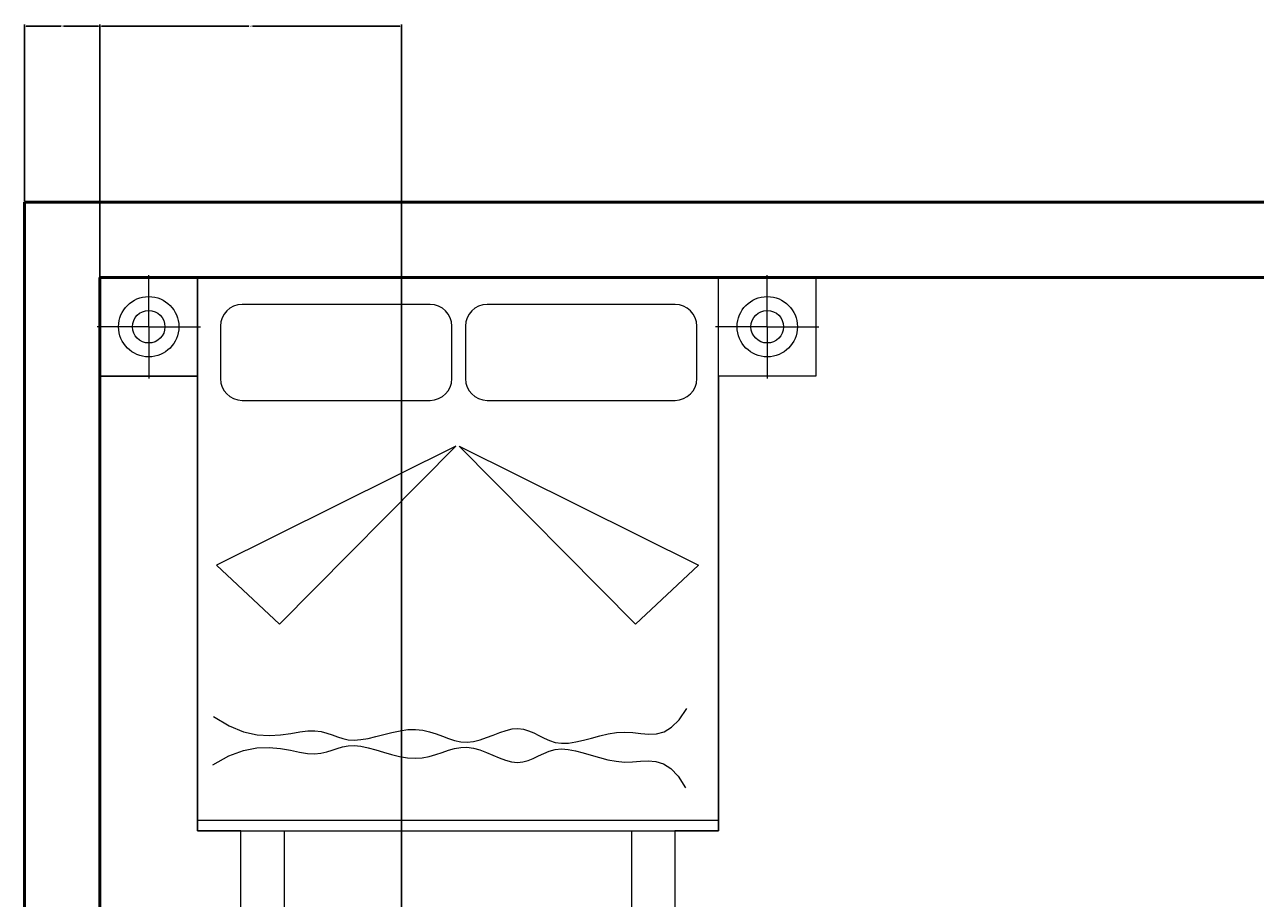
# Model space of a CAD drawing. Units: inches. Extents: x 1798 to 2141, y 1923 to 2386.
# Tile 6 of 9: x 1820 to 1967, y 2281 to 2386. Entities that reach past the tile are written whole.
import ezdxf

# ---------------------------------------------------------------- set-up
doc = ezdxf.new("R2010")
doc.units = ezdxf.units.IN
for name, color, linetype, lineweight in [('A-ANNO-DIMS', 2, 'Continuous', 18), ('A-FURN', 8, 'Continuous', 13), ('wall', 4, 'Continuous', 50)]:
    doc.layers.add(name, color=color, linetype=linetype, lineweight=lineweight)
doc.styles.get("Standard").update_dxf_attribs({"font": 'arial.ttf'})
doc.dimstyles.get("Standard").update_dxf_attribs({"dimtxt": 0.18, "dimasz": 0.18, "dimexe": 0.18, "dimexo": 0.0625, "dimgap": 0.09, "dimtad": 0, "dimtih": 1, "dimtoh": 1, "dimdec": 4, "dimzin": 0, "dimdsep": 46, "dimtxsty": 'Standard', "dimcen": 0.09, "dimadec": 0, "dimazin": 0, "dimtfac": 1, "dimtdec": 4, "dimtofl": 0, "dimtmove": 0, "dimatfit": 3, "dimfxl": 1, "dimtolj": 1, "dimtzin": 0, "dimarcsym": 0})

# ---------------------------------------------------------------- blocks, each defined once
blk = doc.blocks.new('A$C4F543DC7')
for p, q in [((0.0134, 3.35, -0.1688), (3.3134, 3.35, -0.1688)), ((0.4634, 3.35, -0.1688), (0.0134, 3.35, -0.1688)), ((0.0134, 2.896, -0.1688), (0.0134, 3.35, -0.1688)), ((0.0134, 3.35, -0.1688), (0.0134, 2.896, -0.1688)), ((0.2381, 3.1233, -0.4388), (0.2381, 3.3614, -0.4388)), ((0.4634, 3.35, -0.1688), (0.4634, 0.8, -0.1688)), ((2.8634, 3.35, -0.1688), (0.4634, 3.35, -0.1688)), ((0.4634, 2.896, -0.1688), (0.4634, 3.35, -0.1688)), ((2.8634, 0.8, -0.1688), (2.8634, 3.35, -0.1688)), ((2.8634, 3.35, -0.1688), (3.3134, 3.35, -0.1688)), ((2.8634, 2.896, -0.1688), (2.8634, 3.35, -0.1688)), ((3.0888, 3.1233, -0.4388), (3.0888, 3.3614, -0.4388)), ((3.3134, 3.35, -0.1688), (3.3134, 2.896, -0.1688)), ((3.3134, 3.35, -0.1688), (3.3134, 2.896, -0.1688)), ((1.5354, 3.226, -0.1688), (0.6684, 3.226, -0.1688)), ((2.6644, 3.226, -0.1688), (1.7974, 3.226, -0.1688)), ((0.2381, 3.1233, -0.4388), (0, 3.1233, -0.4388)), ((0.2381, 3.1233, -0.4388), (0.4762, 3.1233, -0.4388)), ((0.2381, 3.1233, -0.4388), (0.2381, 2.8852, -0.4388)), ((0.5684, 3.126, -0.1688), (0.5684, 2.884, -0.1688)), ((1.6354, 2.884, -0.1688), (1.6354, 3.126, -0.1688)), ((1.6974, 3.126, -0.1688), (1.6974, 2.884, -0.1688)), ((2.7644, 2.884, -0.1688), (2.7644, 3.126, -0.1688)), ((3.0888, 3.1233, -0.4388), (2.8507, 3.1233, -0.4388)), ((3.0888, 3.1233, -0.4388), (3.0888, 2.8852, -0.4388)), ((3.0888, 3.1233, -0.4388), (3.3269, 3.1233, -0.4388)), ((0.4634, 2.896, -0.1688), (0.0134, 2.896, -0.1688)), ((0.0134, 2.896, -0.1688), (0.4634, 2.896, -0.1688)), ((0.4634, 0.8, -0.1688), (0.4634, 2.896, -0.1688)), ((2.8634, 2.896, -0.1688), (2.8634, 0.8, -0.1688)), ((3.3134, 2.896, -0.1688), (2.8634, 2.896, -0.1688)), ((3.3134, 2.896, -0.1688), (2.8634, 2.896, -0.1688)), ((0.6684, 2.784, -0.1688), (1.5354, 2.784, -0.1688)), ((1.7974, 2.784, -0.1688), (2.6644, 2.784, -0.1688)), ((1.6534, 2.573, -0.1688), (0.5504, 2.025, -0.1688)), ((0.8414, 1.752, -0.1688), (1.6534, 2.573, -0.1688)), ((2.4814, 1.752, -0.1688), (1.6694, 2.573, -0.1688)), ((1.6694, 2.573, -0.1688), (2.7724, 2.025, -0.1688)), ((0.5504, 2.025, -0.1688), (0.8414, 1.752, -0.1688)), ((2.7724, 2.025, -0.1688), (2.4814, 1.752, -0.1688)), ((2.683, 1.312, -0.1688), (2.7182, 1.3641, -0.1688)), ((0.5369, 1.3267, -0.1688), (0.6088, 1.2835, -0.1688)), ((2.6479, 1.2774, -0.1688), (2.683, 1.312, -0.1688)), ((0.6088, 1.2835, -0.1688), (0.6756, 1.2566, -0.1688)), ((0.6756, 1.2566, -0.1688), (0.7373, 1.2428, -0.1688)), ((0.8457, 1.242, -0.1688), (0.8925, 1.2489, -0.1688)), ((0.8925, 1.2489, -0.1688), (0.9345, 1.2564, -0.1688)), ((0.9345, 1.2564, -0.1688), (0.9718, 1.2615, -0.1688)), ((0.9718, 1.2615, -0.1688), (1.0044, 1.2617, -0.1688)), ((1.0044, 1.2617, -0.1688), (1.0334, 1.2578, -0.1688)), ((1.0334, 1.2578, -0.1688), (1.0597, 1.2509, -0.1688)), ((1.0597, 1.2509, -0.1688), (1.0842, 1.2424, -0.1688)), ((1.3218, 1.2441, -0.1688), (1.3591, 1.2533, -0.1688)), ((1.3591, 1.2533, -0.1688), (1.3963, 1.2612, -0.1688)), ((1.3963, 1.2612, -0.1688), (1.4328, 1.2664, -0.1688)), ((1.4328, 1.2664, -0.1688), (1.4679, 1.2677, -0.1688)), ((1.4679, 1.2677, -0.1688), (1.501, 1.2643, -0.1688)), ((1.501, 1.2643, -0.1688), (1.5324, 1.257, -0.1688)), ((1.5324, 1.257, -0.1688), (1.5624, 1.2473, -0.1688)), ((1.8258, 1.2417, -0.1688), (1.8557, 1.2531, -0.1688)), ((1.8557, 1.2531, -0.1688), (1.8849, 1.263, -0.1688)), ((1.8849, 1.263, -0.1688), (1.913, 1.2698, -0.1688)), ((1.913, 1.2698, -0.1688), (1.9397, 1.2722, -0.1688)), ((1.9397, 1.2722, -0.1688), (1.9649, 1.2692, -0.1688)), ((1.9649, 1.2692, -0.1688), (1.989, 1.2617, -0.1688)), ((1.989, 1.2617, -0.1688), (2.0124, 1.2512, -0.1688)), ((2.0124, 1.2512, -0.1688), (2.0359, 1.2391, -0.1688)), ((2.3558, 1.2465, -0.1688), (2.3944, 1.2527, -0.1688)), ((2.3944, 1.2527, -0.1688), (2.4325, 1.255, -0.1688)), ((2.4325, 1.255, -0.1688), (2.4698, 1.2529, -0.1688)), ((2.4698, 1.2529, -0.1688), (2.5064, 1.2488, -0.1688)), ((2.5064, 1.2488, -0.1688), (2.5423, 1.2459, -0.1688)), ((2.5777, 1.2476, -0.1688), (2.6129, 1.257, -0.1688)), ((2.6129, 1.257, -0.1688), (2.6479, 1.2774, -0.1688)), ((0.7373, 1.2428, -0.1688), (0.794, 1.239, -0.1688)), ((0.794, 1.239, -0.1688), (0.8457, 1.242, -0.1688)), ((1.0842, 1.2424, -0.1688), (1.1081, 1.2336, -0.1688)), ((1.1081, 1.2336, -0.1688), (1.1322, 1.2257, -0.1688)), ((1.1316, 1.1872, -0.1688), (1.1573, 1.192, -0.1688)), ((1.1322, 1.2257, -0.1688), (1.1577, 1.2201, -0.1688)), ((1.1573, 1.192, -0.1688), (1.1851, 1.1932, -0.1688)), ((1.1577, 1.2201, -0.1688), (1.1855, 1.218, -0.1688)), ((1.1851, 1.1932, -0.1688), (1.2158, 1.1898, -0.1688)), ((1.1855, 1.218, -0.1688), (1.2163, 1.2204, -0.1688)), ((1.2163, 1.2204, -0.1688), (1.2498, 1.2264, -0.1688)), ((1.2498, 1.2264, -0.1688), (1.2852, 1.2347, -0.1688)), ((1.2852, 1.2347, -0.1688), (1.3218, 1.2441, -0.1688)), ((1.5624, 1.2473, -0.1688), (1.5915, 1.2365, -0.1688)), ((1.5915, 1.2365, -0.1688), (1.6199, 1.2259, -0.1688)), ((1.6199, 1.2259, -0.1688), (1.6481, 1.2169, -0.1688)), ((1.6481, 1.2169, -0.1688), (1.6765, 1.2108, -0.1688)), ((1.6765, 1.2108, -0.1688), (1.7053, 1.209, -0.1688)), ((1.7053, 1.209, -0.1688), (1.7349, 1.2124, -0.1688)), ((1.7349, 1.2124, -0.1688), (1.7651, 1.2199, -0.1688)), ((1.7651, 1.2199, -0.1688), (1.7955, 1.2301, -0.1688)), ((1.7955, 1.2301, -0.1688), (1.8258, 1.2417, -0.1688)), ((2.0359, 1.2391, -0.1688), (2.0599, 1.2269, -0.1688)), ((2.0599, 1.2269, -0.1688), (2.0849, 1.216, -0.1688)), ((2.0849, 1.216, -0.1688), (2.1117, 1.2077, -0.1688)), ((2.1117, 1.2077, -0.1688), (2.1407, 1.2037, -0.1688)), ((2.1407, 1.2037, -0.1688), (2.1723, 1.2047, -0.1688)), ((2.1723, 1.2047, -0.1688), (2.2062, 1.21, -0.1688)), ((2.2062, 1.21, -0.1688), (2.242, 1.2182, -0.1688)), ((2.242, 1.2182, -0.1688), (2.2791, 1.2279, -0.1688)), ((2.2791, 1.2279, -0.1688), (2.3173, 1.2378, -0.1688)), ((2.3173, 1.2378, -0.1688), (2.3558, 1.2465, -0.1688)), ((2.5423, 1.2459, -0.1688), (2.5777, 1.2476, -0.1688)), ((0.5334, 1.105, -0.1688), (0.6067, 1.1458, -0.1688)), ((0.6067, 1.1458, -0.1688), (0.6743, 1.1706, -0.1688)), ((0.6743, 1.1706, -0.1688), (0.7364, 1.1825, -0.1688)), ((0.7364, 1.1825, -0.1688), (0.7931, 1.1846, -0.1688)), ((0.7931, 1.1846, -0.1688), (0.8447, 1.1799, -0.1688)), ((0.8447, 1.1799, -0.1688), (0.8913, 1.1716, -0.1688)), ((0.8913, 1.1716, -0.1688), (0.9331, 1.1628, -0.1688)), ((0.9331, 1.1628, -0.1688), (0.9701, 1.1565, -0.1688)), ((0.9701, 1.1565, -0.1688), (1.0027, 1.1552, -0.1688)), ((1.0027, 1.1552, -0.1688), (1.0318, 1.1582, -0.1688)), ((1.0318, 1.1582, -0.1688), (1.0583, 1.1642, -0.1688)), ((1.0583, 1.1642, -0.1688), (1.0831, 1.172, -0.1688)), ((1.0831, 1.172, -0.1688), (1.1072, 1.18, -0.1688)), ((1.1072, 1.18, -0.1688), (1.1316, 1.1872, -0.1688)), ((1.2158, 1.1898, -0.1688), (1.2491, 1.1828, -0.1688)), ((1.2491, 1.1828, -0.1688), (1.2842, 1.1734, -0.1688)), ((1.2842, 1.1734, -0.1688), (1.3206, 1.1629, -0.1688)), ((1.3206, 1.1629, -0.1688), (1.3575, 1.1524, -0.1688)), ((1.3575, 1.1524, -0.1688), (1.3945, 1.1434, -0.1688)), ((1.3945, 1.1434, -0.1688), (1.4308, 1.1371, -0.1688)), ((1.4308, 1.1371, -0.1688), (1.4658, 1.1347, -0.1688)), ((1.4658, 1.1347, -0.1688), (1.499, 1.137, -0.1688)), ((1.499, 1.137, -0.1688), (1.5306, 1.1433, -0.1688)), ((1.5306, 1.1433, -0.1688), (1.5609, 1.152, -0.1688)), ((1.5609, 1.152, -0.1688), (1.5903, 1.1619, -0.1688)), ((1.5903, 1.1619, -0.1688), (1.6191, 1.1716, -0.1688)), ((1.6191, 1.1716, -0.1688), (1.6475, 1.1797, -0.1688)), ((1.6475, 1.1797, -0.1688), (1.676, 1.1849, -0.1688)), ((1.676, 1.1849, -0.1688), (1.7049, 1.1858, -0.1688)), ((1.7049, 1.1858, -0.1688), (1.7344, 1.1816, -0.1688)), ((1.7344, 1.1816, -0.1688), (1.7643, 1.1731, -0.1688)), ((1.7643, 1.1731, -0.1688), (1.7944, 1.1619, -0.1688)), ((1.7944, 1.1619, -0.1688), (1.8244, 1.1494, -0.1688)), ((1.8244, 1.1494, -0.1688), (1.8539, 1.137, -0.1688)), ((1.8539, 1.137, -0.1688), (1.8827, 1.1263, -0.1688)), ((2.0106, 1.134, -0.1688), (2.0344, 1.1454, -0.1688)), ((2.0344, 1.1454, -0.1688), (2.0588, 1.1568, -0.1688)), ((2.0588, 1.1568, -0.1688), (2.0842, 1.167, -0.1688)), ((2.0842, 1.167, -0.1688), (2.1112, 1.1743, -0.1688)), ((2.1112, 1.1743, -0.1688), (2.1403, 1.1775, -0.1688)), ((2.1403, 1.1775, -0.1688), (2.1718, 1.1755, -0.1688)), ((2.1718, 1.1755, -0.1688), (2.2056, 1.1691, -0.1688)), ((2.2056, 1.1691, -0.1688), (2.2411, 1.1598, -0.1688)), ((2.2411, 1.1598, -0.1688), (2.2779, 1.1489, -0.1688)), ((2.2779, 1.1489, -0.1688), (2.3157, 1.1379, -0.1688)), ((2.3157, 1.1379, -0.1688), (2.354, 1.1279, -0.1688)), ((1.8827, 1.1263, -0.1688), (1.9106, 1.1186, -0.1688)), ((1.9106, 1.1186, -0.1688), (1.9373, 1.1153, -0.1688)), ((1.9373, 1.1153, -0.1688), (1.9625, 1.1176, -0.1688)), ((1.9625, 1.1176, -0.1688), (1.9868, 1.1243, -0.1688)), ((1.9868, 1.1243, -0.1688), (2.0106, 1.134, -0.1688)), ((2.354, 1.1279, -0.1688), (2.3923, 1.1205, -0.1688)), ((2.3923, 1.1205, -0.1688), (2.4304, 1.117, -0.1688)), ((2.4304, 1.117, -0.1688), (2.4677, 1.118, -0.1688)), ((2.4677, 1.118, -0.1688), (2.5043, 1.1209, -0.1688)), ((2.5043, 1.1209, -0.1688), (2.5403, 1.1226, -0.1688)), ((2.5403, 1.1226, -0.1688), (2.5757, 1.1199, -0.1688)), ((2.5757, 1.1199, -0.1688), (2.6106, 1.1094, -0.1688)), ((2.6106, 1.1094, -0.1688), (2.645, 1.0879, -0.1688)), ((2.645, 1.0879, -0.1688), (2.6789, 1.0522, -0.1688)), ((2.6789, 1.0522, -0.1688), (2.7124, 0.999, -0.1688)), ((0.4634, 0.85, -0.1688), (2.8634, 0.85, -0.1688)), ((0.4634, 0.8, -0.1688), (2.8634, 0.8, -0.1688)), ((0.6634, 0.8, -0.1688), (0.4634, 0.8, -0.1688)), ((0.6634, 0.8, -0.1688), (2.6634, 0.8, -0.1688)), ((0.6634, 0.104, -0.1688), (0.6634, 0.8, -0.1688)), ((0.6634, 0.104, -0.1688), (0.6634, 0.8, -0.1688)), ((0.8634, 0.281, -0.1688), (0.8634, 0.8, -0.1688)), ((2.4634, 0.8, -0.1688), (2.4634, 0.281, -0.1688)), ((2.8634, 0.8, -0.1688), (2.6634, 0.8, -0.1688)), ((2.6634, 0.8, -0.1688), (2.6634, 0.104, -0.1688)), ((2.6634, 0.8, -0.1688), (2.6634, 0.104, -0.1688))]:
    blk.add_line(p, q)
for centre, radius in [((0.2381, 3.1233, -0.4388), 0.139), ((3.0888, 3.1233, -0.4388), 0.139), ((0.2381, 3.1233, -0.4388), 0.075), ((3.0888, 3.1233, -0.4388), 0.075)]:
    blk.add_circle(centre, radius)
for centre, radius, start, end in [((0.6684, 3.126, -0.1688), 0.1, 90, 180), ((1.5354, 3.126, -0.1688), 0.1, 0, 90), ((1.7974, 3.126, -0.1688), 0.1, 90, 180), ((2.6644, 3.126, -0.1688), 0.1, 0, 90), ((0.6684, 2.884, -0.1688), 0.1, 180, 270), ((1.5354, 2.884, -0.1688), 0.1, 270, 0), ((1.7974, 2.884, -0.1688), 0.1, 180, 270), ((2.6644, 2.884, -0.1688), 0.1, 270, 0), ((0.6994, 0.3472, -0.1688), 0.1769, 258.2616, 338.032), ((2.6275, 0.3472, -0.1688), 0.1769, 201.968, 281.7384), ((1.6634, 4.8597, -0.1688), 4.8597, 258.1252, 281.8748), ((1.6634, 4.8597, -0.1688), 4.8597, 258.1252, 281.8748)]:
    blk.add_arc(centre, radius, start, end)
blk = doc.blocks.new('*D33')
at = {"layer": 'A-ANNO-DIMS', "color": 0, "lineweight": -2, "transparency": 16777216}
for p, q in [((1819.51, 2364.39), (1819.51, 2385.53)), ((1819.69, 2385.35), (1823.86, 2385.35)), ((1828.33, 2385.35), (1824.16, 2385.35)), ((1828.51, 2355.39), (1828.51, 2385.53))]:
    blk.add_line(p, q, dxfattribs=at)
at = {"layer": 'A-ANNO-DIMS', "color": 0, "transparency": 16777216}
for points in [[(1819.69, 2385.38), (1819.69, 2385.32), (1819.51, 2385.35)], [(1828.33, 2385.38), (1828.33, 2385.32), (1828.51, 2385.35)]]:
    blk.add_solid(points, dxfattribs=at)
at = {"layer": 'Defpoints', "color": 0, "transparency": 16777216}
for p in [(1828.51, 2385.35), (1819.51, 2364.32), (1828.51, 2355.32)]:
    blk.add_point(p, dxfattribs=at)
at = {"layer": 'A-ANNO-DIMS', "color": 0, "transparency": 16777216, "insert": (1824.01, 2385.35), "char_height": 0.18, "attachment_point": 5}
blk.add_mtext('\\A1;9', dxfattribs=at)
blk = doc.blocks.new('*D43')
at = {"layer": 'A-ANNO-DIMS', "color": 0, "lineweight": -2, "transparency": 16777216}
for p, q in [((1828.51, 2174.39), (1828.51, 2385.53)), ((1828.69, 2385.35), (1846.3, 2385.35)), ((1864.33, 2385.35), (1846.73, 2385.35)), ((1864.51, 2174.39), (1864.51, 2385.53))]:
    blk.add_line(p, q, dxfattribs=at)
at = {"layer": 'A-ANNO-DIMS', "color": 0, "transparency": 16777216}
for points in [[(1828.69, 2385.38), (1828.69, 2385.32), (1828.51, 2385.35)], [(1864.33, 2385.38), (1864.33, 2385.32), (1864.51, 2385.35)]]:
    blk.add_solid(points, dxfattribs=at)
at = {"layer": 'Defpoints', "color": 0, "transparency": 16777216}
for p in [(1864.51, 2385.35), (1828.51, 2174.32), (1864.51, 2174.32)]:
    blk.add_point(p, dxfattribs=at)
at = {"layer": 'A-ANNO-DIMS', "color": 0, "transparency": 16777216, "insert": (1846.51, 2385.35), "char_height": 0.18, "attachment_point": 5}
blk.add_mtext('\\A1;36', dxfattribs=at)

msp = doc.modelspace()

# ---------------------------------------------------------------- linework, layer by layer
at = {"layer": 'wall'}
for p, q in [((2119.5141, 2364.3239), (1819.5141, 2364.3239)), ((1819.5141, 2364.3239), (1819.5141, 1944.3239)), ((2110.5141, 2355.3239), (1828.5141, 2355.3239)), ((1828.5141, 2355.3239), (1828.5141, 1953.3239))]:
    msp.add_line(p, q, dxfattribs=at)

# ---------------------------------------------------------------- block references
at = {"layer": 'A-FURN', "xscale": 25.91562772622874, "yscale": 25.91562772622874, "zscale": 25.91562772622874}
msp.add_blockref('A$C4F543DC7', (1828.1659, 2268.5065, 4.3733), dxfattribs=at)

# ---------------------------------------------------------------- dimensions: what is measured, and where the dimension line sits
at = {"layer": 'A-ANNO-DIMS'}
for base, p1, p2, picture, middle in [((1828.5141, 2385.3489), (1819.5141, 2364.3239), (1828.5141, 2355.3239), '*D33', (1824.0141, 2385.3489)), ((1864.5141, 2385.3489), (1828.5141, 2174.3239), (1864.5141, 2174.3239), '*D43', (1846.5141, 2385.3489))]:
    dim = msp.add_linear_dim(base=base, p1=p1, p2=p2, dimstyle='Standard', override={"dimdec": 0, "dimlfac": 1, "dimrnd": 0, "dimzin": 0, "dimdsep": 46, "dimlunit": 2}, dxfattribs=at)
    dim.commit()
    dim.dimension.update_dxf_attribs({"geometry": picture, "text_midpoint": middle})

doc.saveas('drawing.dxf')
